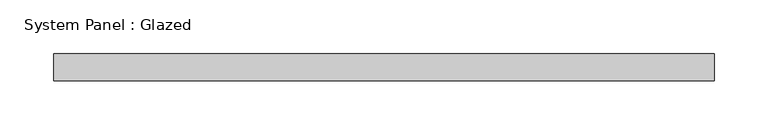
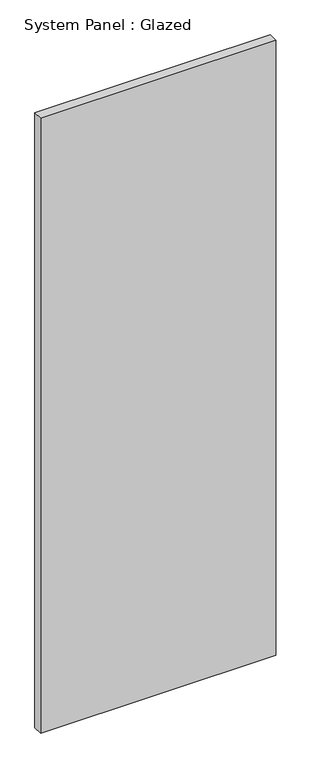
"""IFC4 building model written with IfcOpenShell, lengths in millimetres: plate geometry, System Panel : Glazed."""

from ifc_helpers import new_model, si_unit, origin, origin_with_axes, place, context, project, spatial, polyline, outline, extrude, source, transform, mapped, element, save


def system_panel_glazed_d2c73f4b(model_context):
    return source(origin(), model_context, "Body", "SweptSolid", [
        extrude(outline(polyline([(307.975, 19.05), (-307.975, 19.05), (-307.975, 44.45), (307.975, 44.45), (307.975, 19.05)])), origin_with_axes(), (0.0, 0.0, 1.0), 1701.8),
    ])


if __name__ == "__main__":
    model = new_model("IFC4")
    model_context = context("Model", 3, world=origin())
    ifc_project = project(units=[si_unit("LENGTHUNIT", "METRE", prefix="MILLI")], contexts=[model_context])
    site = spatial("IfcSite", under=ifc_project)
    building = spatial("IfcBuilding", under=site)
    placement = place(None, origin())
    system_panel_glazed_shape = system_panel_glazed_d2c73f4b(model_context)
    element("IfcPlate", 1, ObjectType="System Panel : Glazed", at=placement, inside=building, context=model_context, shape_type="MappedRepresentation", body=[
        mapped(system_panel_glazed_shape, transform((0.0, 0.0, 0.0), x_axis=(1.0, 0.0, 0.0), y_axis=(0.0, 1.0, 0.0), z_axis=(0.0, 0.0, 1.0))),
    ])
    save(model, "model.ifc")

# Revit data of these elements
# Type "System Panel : Glazed"
#   Construction Type Id = "GSP4R"
#   Analytic Construction = "1/8 in Pilkington single glazing"
#   Visual Light Transmittance = 0.9
#   Solar Heat Gain Coefficient = 0.86
#   Heat Transfer Coefficient (U) = 1.18115 BTU/(h·ft²·°F)
#   Define Thermal Properties by = 1
# Element 1 (IfcPlate, "System Panel : Glazed")
#   Materials on its faces: "Glass"
# Materials
#   "Glass": class "Glass", colour RGB 0 128 192, transparency 0.75, Description = "Soda Lime Glass", Cost = 0
